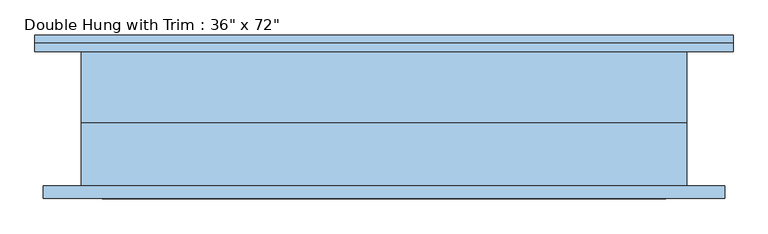
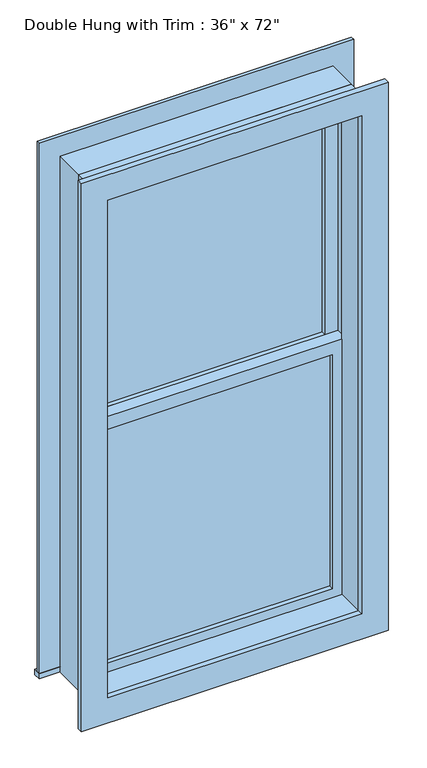
"""IFC4 building model written with IfcOpenShell, lengths in millimetres: window geometry."""

from ifc_helpers import new_model, si_unit, frame, origin, place, context, project, spatial, polyline, outline, extrude, source, transform, mapped, element, save


def window_d3583dd1(model_context):
    return source(origin(), model_context, "Body", "SweptSolid", [
        extrude(outline(polyline([(-393.7, 22.225), (393.7, 22.225), (393.7, 9.525), (-393.7, 9.525), (-393.7, 22.225)])), frame((0.0, 0.0, 368.3), z_axis=(0.0, 0.0, 1.0), x_axis=(1.0, 0.0, 0.0)), (0.0, 0.0, 1.0), 828.675),
        extrude(outline(polyline([(1241.425, -438.15), (323.85, -438.15), (323.85, 438.15), (1241.425, 438.15), (1241.425, -438.15)]), holes=[polyline([(1196.975, -393.7), (1196.975, 393.7), (368.3, 393.7), (368.3, -393.7), (1196.975, -393.7)])]), frame((0.0, -6.35, 0.0), z_axis=(0.0, 1.0, 0.0), x_axis=(0.0, 0.0, 1.0)), (0.0, 0.0, 1.0), 44.45),
        extrude(outline(polyline([(-527.05, 127.0), (527.05, 127.0), (527.05, 101.6), (-527.05, 101.6), (-527.05, 127.0)])), frame((0.0, 0.0, 304.8), z_axis=(0.0, 0.0, 1.0), x_axis=(1.0, 0.0, 0.0)), (0.0, 0.0, 1.0), 19.05),
        extrude(outline(polyline([(2114.55, -438.15), (2114.55, 438.15), (323.85, 438.15), (323.85, 527.05), (2203.45, 527.05), (2203.45, -527.05), (323.85, -527.05), (323.85, -438.15), (2114.55, -438.15)])), frame((0.0, 101.6, 0.0), z_axis=(0.0, 1.0, 0.0), x_axis=(0.0, 0.0, 1.0)), (0.0, 0.0, 1.0), 12.7),
        extrude(outline(polyline([(2190.75, 514.35), (2190.75, -514.35), (247.65, -514.35), (247.65, 514.35), (2190.75, 514.35)]), holes=[polyline([(2101.85, 425.45), (336.55, 425.45), (336.55, -425.45), (2101.85, -425.45), (2101.85, 425.45)])]), frame((0.0, -120.65, 0.0), z_axis=(0.0, 1.0, 0.0), x_axis=(0.0, 0.0, 1.0)), (0.0, 0.0, 1.0), 19.05),
        extrude(outline(polyline([(393.7, 53.975), (-393.7, 53.975), (-393.7, 66.675), (393.7, 66.675), (393.7, 53.975)])), frame((0.0, 0.0, 1241.425), z_axis=(0.0, 0.0, 1.0), x_axis=(1.0, 0.0, 0.0)), (0.0, 0.0, 1.0), 828.675),
        extrude(outline(polyline([(2114.55, -438.15), (1196.975, -438.15), (1196.975, 438.15), (2114.55, 438.15), (2114.55, -438.15)]), holes=[polyline([(2070.1, -393.7), (2070.1, 393.7), (1241.425, 393.7), (1241.425, -393.7), (2070.1, -393.7)])]), frame((0.0, 38.1, 0.0), z_axis=(0.0, 1.0, 0.0), x_axis=(0.0, 0.0, 1.0)), (0.0, 0.0, 1.0), 44.45),
        extrude(outline(polyline([(2133.6, -457.2), (304.8, -457.2), (304.8, 457.2), (2133.6, 457.2), (2133.6, -457.2)]), holes=[polyline([(2101.85, -425.45), (2101.85, 425.45), (336.55, 425.45), (336.55, -425.45), (2101.85, -425.45)])]), frame((0.0, -101.6, 0.0), z_axis=(0.0, 1.0, 0.0), x_axis=(0.0, 0.0, 1.0)), (0.0, 0.0, 1.0), 95.25),
        extrude(outline(polyline([(2133.6, 457.2), (2133.6, -457.2), (304.8, -457.2), (304.8, 457.2), (2133.6, 457.2)]), holes=[polyline([(2114.55, 438.15), (323.85, 438.15), (323.85, -438.15), (2114.55, -438.15), (2114.55, 438.15)])]), frame((0.0, -6.35, 0.0), z_axis=(0.0, 1.0, 0.0), x_axis=(0.0, 0.0, 1.0)), (0.0, 0.0, 1.0), 107.95),
    ])


if __name__ == "__main__":
    model = new_model("IFC4")
    model_context = context("Model", 3, world=origin())
    ifc_project = project(units=[si_unit("LENGTHUNIT", "METRE", prefix="MILLI")], contexts=[model_context])
    site = spatial("IfcSite", under=ifc_project)
    building = spatial("IfcBuilding", under=site)
    placement = place(None, origin())
    window_shape = window_d3583dd1(model_context)
    element("IfcWindow", 1, ObjectType="Double Hung with Trim : 36\" x 72\"", at=placement, inside=building, context=model_context, shape_type="MappedRepresentation", body=[
        mapped(window_shape, transform((0.0, 0.0, 0.0), x_axis=(1.0, 0.0, 0.0), y_axis=(0.0, 1.0, 0.0), z_axis=(0.0, 0.0, 1.0))),
    ])
    save(model, "model.ifc")

# Revit data of these elements
# Type "Double Hung with Trim : 36\" x 72\""
#   Type Mark = "18"
#   Construction Type Id = "GSP4R"
#   Assembly Code = "B2020100"
#   Analytic Construction = "1/8 in Pilkington single glazing"
#   Visual Light Transmittance = 0.9
#   Solar Heat Gain Coefficient = 0.78
#   Heat Transfer Coefficient (U) = 0.6496 BTU/(h·ft²·°F)
#   Height = 6' - 0"
#   Default Sill Height = 1' - 0"
#   Trim Projection - Ext. = 0' - 0 1/2"
#   Trim Projection - Int. = 0' - 0 3/4"
#   Trim Width - Exterior = 0' - 3 1/2"
#   Trim Width - Interior = 0' - 3 1/2"
#   Width = 3' - 0"
#   Window Inset = 0' - 0 3/4"
#   Define Thermal Properties by = 1
#   Glass Pane Material = Glass
#   Sash Material = Sash
#   Trim Exterior Material = Trim
#   Trim Interior Material = Trim
#   Wall Closure = (empty or 0)
# Element 1 (IfcWindow, "Double Hung with Trim : 36\" x 72\"")
#   Materials on its faces: "Sash", "Trim", "Glass"
# Materials
#   "Glass": class "Glass", colour RGB 0 128 192, transparency 0.75, Description = "Soda Lime Glass", Cost = 0
#   "Sash": class "Wood", colour RGB 224 178 126, transparency 0
#   "Trim": class "Wood", colour RGB 224 178 126, transparency 0
